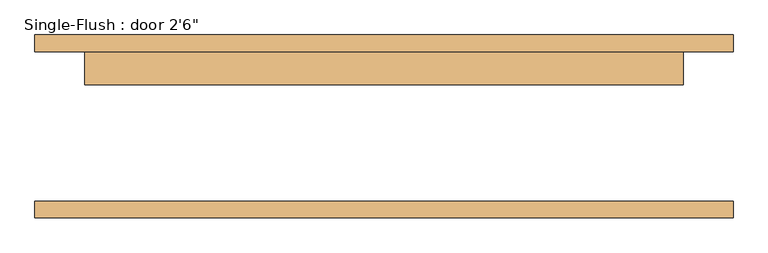
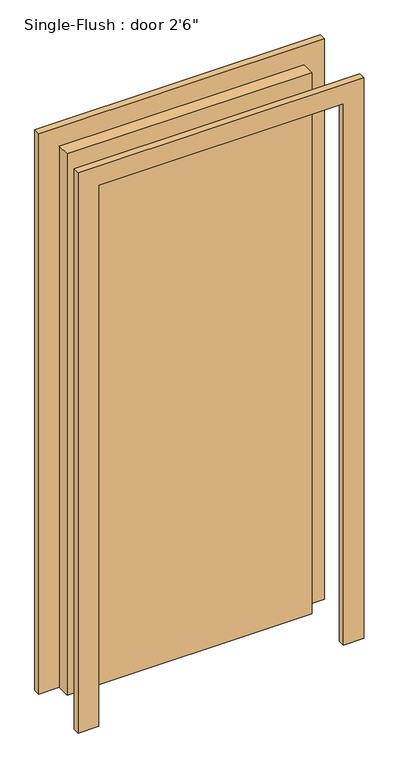
"""IFC4 building model written with IfcOpenShell, lengths in millimetres: door geometry."""

from ifc_helpers import new_model, si_unit, frame, origin, origin_with_axes, place, context, project, spatial, polyline, outline, extrude, source, transform, mapped, element, save


def door_0ca8825f(model_context):
    return source(origin(), model_context, "Body", "SweptSolid", [
        extrude(outline(polyline([(2209.8, -533.4), (0.0, -533.4), (0.0, -457.2), (2133.6, -457.2), (2133.6, 457.2), (0.0, 457.2), (0.0, 533.4), (2209.8, 533.4), (2209.8, -533.4)])), frame((0.0, 114.3, 0.0), z_axis=(0.0, 1.0, 0.0), x_axis=(0.0, 0.0, 1.0)), (0.0, 0.0, 1.0), 25.4),
        extrude(outline(polyline([(2209.8, 533.4), (2209.8, -533.4), (0.0, -533.4), (0.0, -457.2), (2133.6, -457.2), (2133.6, 457.2), (0.0, 457.2), (0.0, 533.4), (2209.8, 533.4)])), frame((0.0, -139.7, 0.0), z_axis=(0.0, 1.0, 0.0), x_axis=(0.0, 0.0, 1.0)), (0.0, 0.0, 1.0), 25.4),
        extrude(outline(polyline([(457.2, 63.5), (-457.2, 63.5), (-457.2, 114.3), (457.2, 114.3), (457.2, 63.5)])), origin_with_axes(), (0.0, 0.0, 1.0), 2133.6),
    ])


if __name__ == "__main__":
    model = new_model("IFC4")
    model_context = context("Model", 3, world=origin())
    ifc_project = project(units=[si_unit("LENGTHUNIT", "METRE", prefix="MILLI")], contexts=[model_context])
    site = spatial("IfcSite", under=ifc_project)
    building = spatial("IfcBuilding", under=site)
    placement = place(None, origin())
    door_shape = door_0ca8825f(model_context)
    element("IfcDoor", 1, ObjectType="Single-Flush : door 2'6\"", at=placement, inside=building, context=model_context, shape_type="MappedRepresentation", body=[
        mapped(door_shape, transform((0.0, 0.0, 0.0), x_axis=(1.0, 0.0, 0.0), y_axis=(0.0, 1.0, 0.0), z_axis=(0.0, 0.0, 1.0))),
    ])
    save(model, "model.ifc")

# Revit data of these elements
# Type "Single-Flush : door 2'6\""
#   Type Mark = "8"
#   Construction Type Id = "MDOOR"
#   Assembly Code = "C1020"
#   Analytic Construction = "Metal"
#   Thickness = 0' - 2"
#   Heat Transfer Coefficient (U) = 0.651978 BTU/(h·ft²·°F)
#   Height = 7' - 0"
#   Trim Projection Ext = 0' - 1"
#   Trim Projection Int = 0' - 1"
#   Trim Width = 0' - 3"
#   Width = 3' - 0"
#   Define Thermal Properties by = 1
#   Door Material = Door - Panel
#   Frame Material = Door - Frame
#   Visual Light Transmittance = 0
#   Solar Heat Gain Coefficient = 0
#   Function = (empty or 0)
#   Wall Closure = (empty or 0)
# Element 1 (IfcDoor, "Single-Flush : door 2'6\"")
#   Materials on its faces: "Door - Frame", "Door - Panel"
# Materials
#   "Door - Panel": class "Wood", colour RGB 210 159 95, transparency 0, Cost = 0
#   "Door - Frame": colour RGB 118 70 51, transparency 0, Cost = 0
